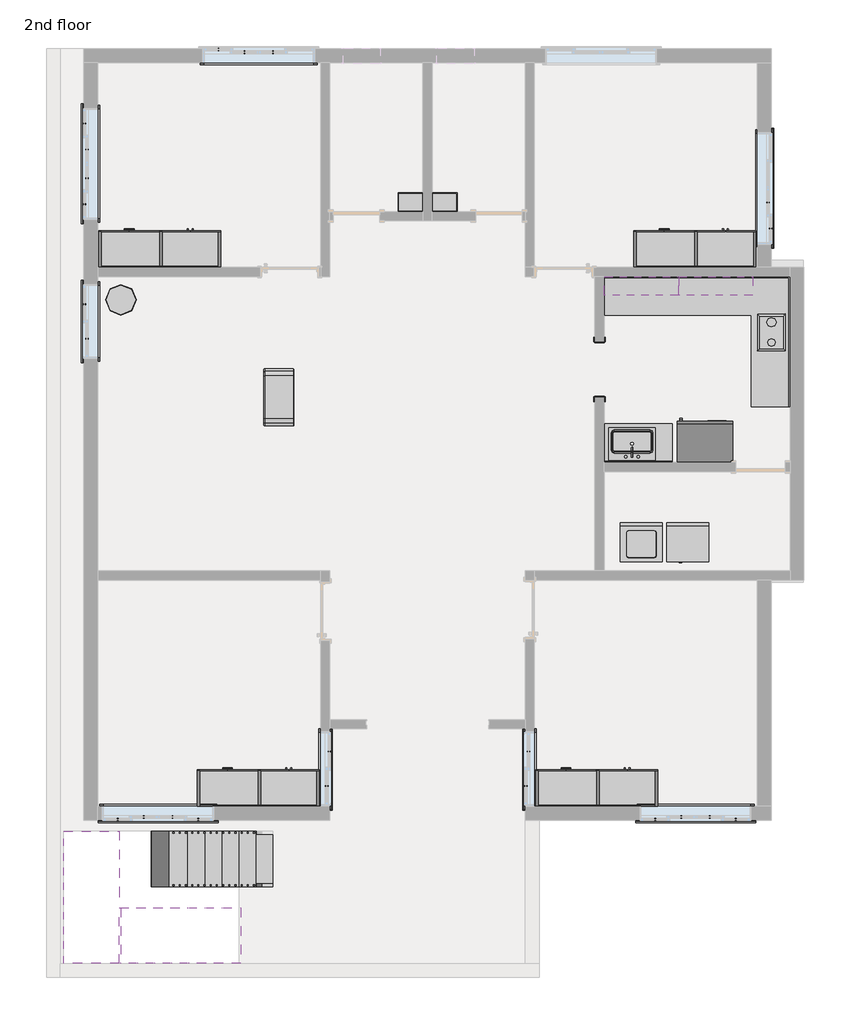
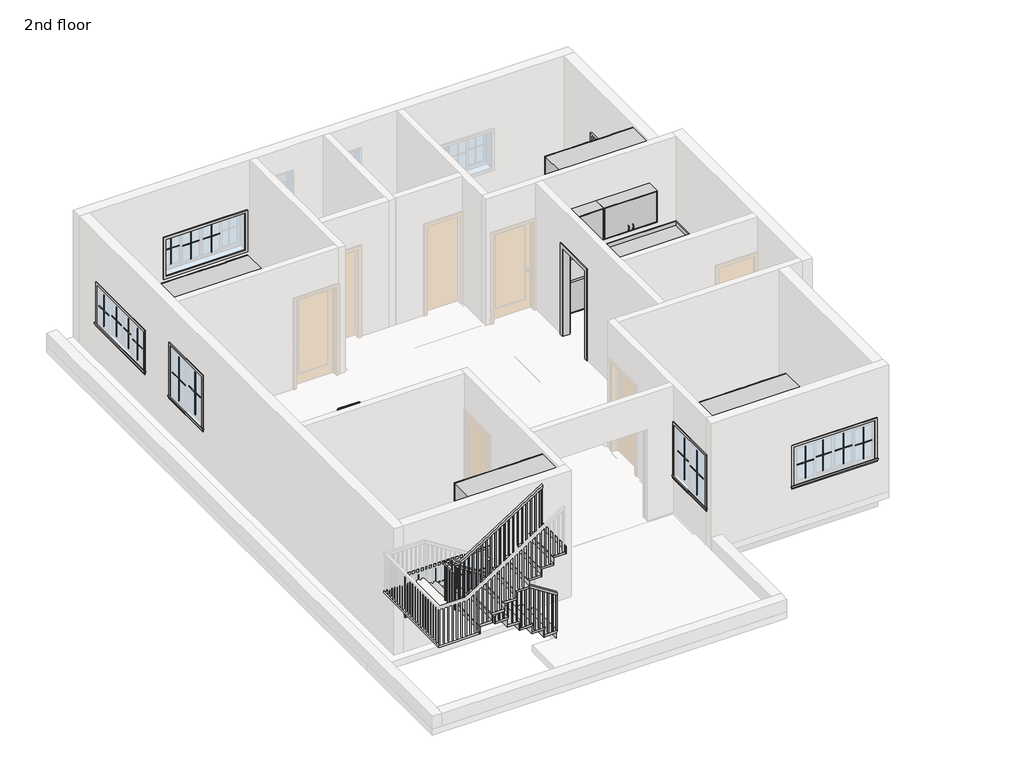
# One storey, part 3 of 4: 42 proxies, 15 furniture elements, 3 flow terminals, 2 stair flights, 1 railing, 1 slab.
"""IFC4 building model written with IfcOpenShell, lengths in millimetres."""

from ifc_helpers import new_model, si_unit, frame, origin, place, context, project, spatial, polyline, outline, extrude, faceted_brep, transform, mapped, element, save
from components import proxy_3c1fa1d0, proxy_97c73763, muntin_pattern_2x2_muntin_pattern_2x2_c2d27229, muntin_pattern_2x2_muntin_pattern_2x2_cf37b409, muntin_pattern_2x2_muntin_pattern_2x2_31a16349, proxy_7dd6dadb, trim_window_exterior_flat_with_sill_ac84ebb5, trim_window_exterior_flat_with_sill_7cfdd449, trim_window_exterior_flat_with_sill_3c945769, trim_window_interior_flat_picture_frame_caf2db4f, trim_window_interior_flat_picture_frame_f1e0b15b, trim_window_interior_flat_picture_frame_0edfbaa2, proxy_e75280ca, flow_terminal_7145266d, flow_terminal_4d548711, furniture_2dca108f, furniture_65fa61b5, furniture_1wardrobe_6271_1wardrobe_6271_4dd35231, furniture_3428e43d, furniture_bf8a676d, furniture_97fe820d, furniture_a6d59748, furniture_f5a42f9b, furniture_9d41381f, furniture_ea954fa4, non_monolithic_landing_bb243dde, stair_flight_4e768039, stair_flight_9d0467a4

model = new_model("IFC4")

# Units and contexts
model_context = context("Model", 3, world=origin())
ifc_project = project(units=[si_unit("LENGTHUNIT", "METRE", prefix="MILLI")], contexts=[model_context])

# Site, building, storey
site = spatial("IfcSite", under=ifc_project)
building = spatial("IfcBuilding", under=site)
storey = spatial("IfcBuildingStorey", under=building, Name="2nd floor", Elevation=7010.4)

# Proxies
placement = place(None, origin())
proxy_shape = proxy_3c1fa1d0(model_context)
element("IfcBuildingElementProxy", 1, Name="Cook Top-2 Unit : 12\" x 18\" 2", ObjectType="Cook Top-2 Unit : 12\" x 18\" 2", at=placement, inside=storey, context=model_context, shape_type="MappedRepresentation", body=[
    mapped(proxy_shape, transform((-1440.8124084, 5502.3713848, 7010.4), x_axis=(1.0, 0.0, 0.0), y_axis=(0.0, 1.0, 0.0), z_axis=(0.0, 0.0, 1.0))),
])
proxy_2_shape = proxy_97c73763(model_context)
element("IfcBuildingElementProxy", 2, Name="Dryer : 27\" x 25\" x 35\"", ObjectType="Dryer : 27\" x 25\" x 35\"", at=placement, inside=storey, context=model_context, shape_type="MappedRepresentation", body=[
    mapped(proxy_2_shape, transform((-3115.1998647, 1776.2351766, 7010.4), x_axis=(1.0, 0.0, 0.0), y_axis=(0.0, 1.0, 0.0), z_axis=(0.0, 0.0, 1.0))),
])
muntin_pattern_2x2_muntin_pattern_2x2_shape = muntin_pattern_2x2_muntin_pattern_2x2_c2d27229(model_context)
element("IfcBuildingElementProxy", 3, Name="Muntin Pattern_2x2 : Muntin Pattern_2x2", ObjectType="Muntin Pattern_2x2 : Muntin Pattern_2x2", at=placement, inside=storey, context=model_context, shape_type="MappedRepresentation", body=[
    mapped(muntin_pattern_2x2_muntin_pattern_2x2_shape, transform((-12588.2374084, 5426.2336804, 8007.35), x_axis=(0.0, -1.0, 0.0), y_axis=(1.0, 0.0, 0.0), z_axis=(0.0, 0.0, 1.0))),
])
element("IfcBuildingElementProxy", 4, Name="Muntin Pattern_2x2 : Muntin Pattern_2x2", ObjectType="Muntin Pattern_2x2 : Muntin Pattern_2x2", at=placement, inside=storey, context=model_context, shape_type="MappedRepresentation", body=[
    mapped(muntin_pattern_2x2_muntin_pattern_2x2_shape, transform((-12632.6874084, 5994.5586804, 8007.35), x_axis=(0.0, -1.0, 0.0), y_axis=(1.0, 0.0, 0.0), z_axis=(0.0, 0.0, 1.0))),
])
muntin_pattern_2x2_muntin_pattern_2x2_2_shape = muntin_pattern_2x2_muntin_pattern_2x2_cf37b409(model_context)
element("IfcBuildingElementProxy", 5, Name="Muntin Pattern_2x2 : Muntin Pattern_2x2", ObjectType="Muntin Pattern_2x2 : Muntin Pattern_2x2", at=placement, inside=storey, context=model_context, shape_type="MappedRepresentation", body=[
    mapped(muntin_pattern_2x2_muntin_pattern_2x2_2_shape, transform((-8657.5874084, -1908.0163196, 8007.35), x_axis=(0.0, -1.0, 0.0), y_axis=(1.0, 0.0, 0.0), z_axis=(0.0, 0.0, 1.0))),
])
element("IfcBuildingElementProxy", 6, Name="Muntin Pattern_2x2 : Muntin Pattern_2x2", ObjectType="Muntin Pattern_2x2 : Muntin Pattern_2x2", at=placement, inside=storey, context=model_context, shape_type="MappedRepresentation", body=[
    mapped(muntin_pattern_2x2_muntin_pattern_2x2_2_shape, transform((-8613.1374084, -1339.6913196, 8007.35), x_axis=(0.0, -1.0, 0.0), y_axis=(1.0, 0.0, 0.0), z_axis=(0.0, 0.0, 1.0))),
])
element("IfcBuildingElementProxy", 7, Name="Muntin Pattern_2x2 : Muntin Pattern_2x2", ObjectType="Muntin Pattern_2x2 : Muntin Pattern_2x2", at=placement, inside=storey, context=model_context, shape_type="MappedRepresentation", body=[
    mapped(muntin_pattern_2x2_muntin_pattern_2x2_2_shape, transform((-5349.2374084, -1339.6913196, 8007.35), x_axis=(0.0, 1.0, 0.0), y_axis=(-1.0, 0.0, 0.0), z_axis=(0.0, 0.0, 1.0))),
])
element("IfcBuildingElementProxy", 8, Name="Muntin Pattern_2x2 : Muntin Pattern_2x2", ObjectType="Muntin Pattern_2x2 : Muntin Pattern_2x2", at=placement, inside=storey, context=model_context, shape_type="MappedRepresentation", body=[
    mapped(muntin_pattern_2x2_muntin_pattern_2x2_2_shape, transform((-5393.6874084, -1908.0163196, 8007.35), x_axis=(0.0, 1.0, 0.0), y_axis=(-1.0, 0.0, 0.0), z_axis=(0.0, 0.0, 1.0))),
])
muntin_pattern_2x2_muntin_pattern_2x2_3_shape = muntin_pattern_2x2_muntin_pattern_2x2_31a16349(model_context)
element("IfcBuildingElementProxy", 9, Name="Muntin Pattern_2x2 : Muntin Pattern_2x2", ObjectType="Muntin Pattern_2x2 : Muntin Pattern_2x2", at=placement, inside=storey, context=model_context, shape_type="MappedRepresentation", body=[
    mapped(muntin_pattern_2x2_muntin_pattern_2x2_3_shape, transform((-10432.4124084, 10171.2711804, 8007.35), x_axis=(1.0, 0.0, 0.0), y_axis=(0.0, 1.0, 0.0), z_axis=(0.0, 0.0, 1.0))),
])
element("IfcBuildingElementProxy", 10, Name="Muntin Pattern_2x2 : Muntin Pattern_2x2", ObjectType="Muntin Pattern_2x2 : Muntin Pattern_2x2", at=placement, inside=storey, context=model_context, shape_type="MappedRepresentation", body=[
    mapped(muntin_pattern_2x2_muntin_pattern_2x2_3_shape, transform((-10006.9624084, 10126.8211804, 8007.35), x_axis=(1.0, 0.0, 0.0), y_axis=(0.0, 1.0, 0.0), z_axis=(0.0, 0.0, 1.0))),
])
element("IfcBuildingElementProxy", 11, Name="Muntin Pattern_2x2 : Muntin Pattern_2x2", ObjectType="Muntin Pattern_2x2 : Muntin Pattern_2x2", at=placement, inside=storey, context=model_context, shape_type="MappedRepresentation", body=[
    mapped(muntin_pattern_2x2_muntin_pattern_2x2_3_shape, transform((-9537.0624084, 10126.8211804, 8007.35), x_axis=(1.0, 0.0, 0.0), y_axis=(0.0, 1.0, 0.0), z_axis=(0.0, 0.0, 1.0))),
])
element("IfcBuildingElementProxy", 12, Name="Muntin Pattern_2x2 : Muntin Pattern_2x2", ObjectType="Muntin Pattern_2x2 : Muntin Pattern_2x2", at=placement, inside=storey, context=model_context, shape_type="MappedRepresentation", body=[
    mapped(muntin_pattern_2x2_muntin_pattern_2x2_3_shape, transform((-12632.6874084, 7634.4461804, 8007.35), x_axis=(0.0, 1.0, 0.0), y_axis=(-1.0, 0.0, 0.0), z_axis=(0.0, 0.0, 1.0))),
])
element("IfcBuildingElementProxy", 13, Name="Muntin Pattern_2x2 : Muntin Pattern_2x2", ObjectType="Muntin Pattern_2x2 : Muntin Pattern_2x2", at=placement, inside=storey, context=model_context, shape_type="MappedRepresentation", body=[
    mapped(muntin_pattern_2x2_muntin_pattern_2x2_3_shape, transform((-12588.2374084, 8059.8961804, 8007.35), x_axis=(0.0, 1.0, 0.0), y_axis=(-1.0, 0.0, 0.0), z_axis=(0.0, 0.0, 1.0))),
])
element("IfcBuildingElementProxy", 14, Name="Muntin Pattern_2x2 : Muntin Pattern_2x2", ObjectType="Muntin Pattern_2x2 : Muntin Pattern_2x2", at=placement, inside=storey, context=model_context, shape_type="MappedRepresentation", body=[
    mapped(muntin_pattern_2x2_muntin_pattern_2x2_3_shape, transform((-12588.2374084, 8529.7961804, 8007.35), x_axis=(0.0, 1.0, 0.0), y_axis=(-1.0, 0.0, 0.0), z_axis=(0.0, 0.0, 1.0))),
])
element("IfcBuildingElementProxy", 15, Name="Muntin Pattern_2x2 : Muntin Pattern_2x2", ObjectType="Muntin Pattern_2x2 : Muntin Pattern_2x2", at=placement, inside=storey, context=model_context, shape_type="MappedRepresentation", body=[
    mapped(muntin_pattern_2x2_muntin_pattern_2x2_3_shape, transform((-12632.6874084, 8955.2461804, 8007.35), x_axis=(0.0, 1.0, 0.0), y_axis=(-1.0, 0.0, 0.0), z_axis=(0.0, 0.0, 1.0))),
])
element("IfcBuildingElementProxy", 16, Name="Muntin Pattern_2x2 : Muntin Pattern_2x2", ObjectType="Muntin Pattern_2x2 : Muntin Pattern_2x2", at=placement, inside=storey, context=model_context, shape_type="MappedRepresentation", body=[
    mapped(muntin_pattern_2x2_muntin_pattern_2x2_3_shape, transform((-1418.5874084, 7659.8461804, 8007.35), x_axis=(0.0, -1.0, 0.0), y_axis=(1.0, 0.0, 0.0), z_axis=(0.0, 0.0, 1.0))),
])
element("IfcBuildingElementProxy", 17, Name="Muntin Pattern_2x2 : Muntin Pattern_2x2", ObjectType="Muntin Pattern_2x2 : Muntin Pattern_2x2", at=placement, inside=storey, context=model_context, shape_type="MappedRepresentation", body=[
    mapped(muntin_pattern_2x2_muntin_pattern_2x2_3_shape, transform((-1374.1374084, 7234.3961804, 8007.35), x_axis=(0.0, -1.0, 0.0), y_axis=(1.0, 0.0, 0.0), z_axis=(0.0, 0.0, 1.0))),
])
element("IfcBuildingElementProxy", 18, Name="Muntin Pattern_2x2 : Muntin Pattern_2x2", ObjectType="Muntin Pattern_2x2 : Muntin Pattern_2x2", at=placement, inside=storey, context=model_context, shape_type="MappedRepresentation", body=[
    mapped(muntin_pattern_2x2_muntin_pattern_2x2_3_shape, transform((-1948.8124084, -2458.8788196, 8007.35), x_axis=(-1.0, 0.0, 0.0), y_axis=(0.0, -1.0, 0.0), z_axis=(0.0, 0.0, 1.0))),
])
element("IfcBuildingElementProxy", 19, Name="Muntin Pattern_2x2 : Muntin Pattern_2x2", ObjectType="Muntin Pattern_2x2 : Muntin Pattern_2x2", at=placement, inside=storey, context=model_context, shape_type="MappedRepresentation", body=[
    mapped(muntin_pattern_2x2_muntin_pattern_2x2_3_shape, transform((-2374.2624084, -2414.4288196, 8007.35), x_axis=(-1.0, 0.0, 0.0), y_axis=(0.0, -1.0, 0.0), z_axis=(0.0, 0.0, 1.0))),
])
element("IfcBuildingElementProxy", 20, Name="Muntin Pattern_2x2 : Muntin Pattern_2x2", ObjectType="Muntin Pattern_2x2 : Muntin Pattern_2x2", at=placement, inside=storey, context=model_context, shape_type="MappedRepresentation", body=[
    mapped(muntin_pattern_2x2_muntin_pattern_2x2_3_shape, transform((-2844.1624084, -2414.4288196, 8007.35), x_axis=(-1.0, 0.0, 0.0), y_axis=(0.0, -1.0, 0.0), z_axis=(0.0, 0.0, 1.0))),
])
element("IfcBuildingElementProxy", 21, Name="Muntin Pattern_2x2 : Muntin Pattern_2x2", ObjectType="Muntin Pattern_2x2 : Muntin Pattern_2x2", at=placement, inside=storey, context=model_context, shape_type="MappedRepresentation", body=[
    mapped(muntin_pattern_2x2_muntin_pattern_2x2_3_shape, transform((-3269.6124084, -2458.8788196, 8007.35), x_axis=(-1.0, 0.0, 0.0), y_axis=(0.0, -1.0, 0.0), z_axis=(0.0, 0.0, 1.0))),
])
element("IfcBuildingElementProxy", 22, Name="Muntin Pattern_2x2 : Muntin Pattern_2x2", ObjectType="Muntin Pattern_2x2 : Muntin Pattern_2x2", at=placement, inside=storey, context=model_context, shape_type="MappedRepresentation", body=[
    mapped(muntin_pattern_2x2_muntin_pattern_2x2_3_shape, transform((-10762.6124084, -2458.8788196, 8007.35), x_axis=(-1.0, 0.0, 0.0), y_axis=(0.0, -1.0, 0.0), z_axis=(0.0, 0.0, 1.0))),
])
element("IfcBuildingElementProxy", 23, Name="Muntin Pattern_2x2 : Muntin Pattern_2x2", ObjectType="Muntin Pattern_2x2 : Muntin Pattern_2x2", at=placement, inside=storey, context=model_context, shape_type="MappedRepresentation", body=[
    mapped(muntin_pattern_2x2_muntin_pattern_2x2_3_shape, transform((-11188.0624084, -2414.4288196, 8007.35), x_axis=(-1.0, 0.0, 0.0), y_axis=(0.0, -1.0, 0.0), z_axis=(0.0, 0.0, 1.0))),
])
element("IfcBuildingElementProxy", 24, Name="Muntin Pattern_2x2 : Muntin Pattern_2x2", ObjectType="Muntin Pattern_2x2 : Muntin Pattern_2x2", at=placement, inside=storey, context=model_context, shape_type="MappedRepresentation", body=[
    mapped(muntin_pattern_2x2_muntin_pattern_2x2_3_shape, transform((-11657.9624084, -2414.4288196, 8007.35), x_axis=(-1.0, 0.0, 0.0), y_axis=(0.0, -1.0, 0.0), z_axis=(0.0, 0.0, 1.0))),
])
element("IfcBuildingElementProxy", 25, Name="Muntin Pattern_2x2 : Muntin Pattern_2x2", ObjectType="Muntin Pattern_2x2 : Muntin Pattern_2x2", at=placement, inside=storey, context=model_context, shape_type="MappedRepresentation", body=[
    mapped(muntin_pattern_2x2_muntin_pattern_2x2_3_shape, transform((-12083.4124084, -2458.8788196, 8007.35), x_axis=(-1.0, 0.0, 0.0), y_axis=(0.0, -1.0, 0.0), z_axis=(0.0, 0.0, 1.0))),
])
proxy_3_shape = proxy_7dd6dadb(model_context)
element("IfcBuildingElementProxy", 26, Name="Passage Opening-Cased : 36\" x 84\"", ObjectType="Passage Opening-Cased : 36\" x 84\"", at=placement, inside=storey, context=model_context, shape_type="MappedRepresentation", body=[
    mapped(proxy_3_shape, transform((-4184.0124084, 4931.1848371, 7010.4), x_axis=(0.0, 1.0, 0.0), y_axis=(-1.0, 0.0, 0.0), z_axis=(0.0, 0.0, 1.0))),
])
trim_window_exterior_flat_with_sill_shape = trim_window_exterior_flat_with_sill_ac84ebb5(model_context)
element("IfcBuildingElementProxy", 27, Name="Trim-Window-Exterior-Flat : with Sill", ObjectType="Trim-Window-Exterior-Flat : with Sill", at=placement, inside=storey, context=model_context, shape_type="MappedRepresentation", body=[
    mapped(trim_window_exterior_flat_with_sill_shape, transform((-12642.2124084, 5710.3961804, 9144.0), x_axis=(0.0, 1.0, 0.0), y_axis=(0.0, 0.0, -1.0), z_axis=(-1.0, 0.0, 0.0))),
])
trim_window_exterior_flat_with_sill_2_shape = trim_window_exterior_flat_with_sill_7cfdd449(model_context)
element("IfcBuildingElementProxy", 28, Name="Trim-Window-Exterior-Flat : with Sill", ObjectType="Trim-Window-Exterior-Flat : with Sill", at=placement, inside=storey, context=model_context, shape_type="MappedRepresentation", body=[
    mapped(trim_window_exterior_flat_with_sill_2_shape, transform((-8603.6124084, -1623.8538196, 9144.0), x_axis=(0.0, 1.0, 0.0), y_axis=(0.0, 0.0, 1.0), z_axis=(1.0, 0.0, 0.0))),
])
element("IfcBuildingElementProxy", 29, Name="Trim-Window-Exterior-Flat : with Sill", ObjectType="Trim-Window-Exterior-Flat : with Sill", at=placement, inside=storey, context=model_context, shape_type="MappedRepresentation", body=[
    mapped(trim_window_exterior_flat_with_sill_2_shape, transform((-5403.2124084, -1623.8538196, 9144.0), x_axis=(0.0, -1.0, 0.0), y_axis=(0.0, 0.0, 1.0), z_axis=(-1.0, 0.0, 0.0))),
])
trim_window_exterior_flat_with_sill_3_shape = trim_window_exterior_flat_with_sill_3c945769(model_context)
element("IfcBuildingElementProxy", 30, Name="Trim-Window-Exterior-Flat : with Sill", ObjectType="Trim-Window-Exterior-Flat : with Sill", at=placement, inside=storey, context=model_context, shape_type="MappedRepresentation", body=[
    mapped(trim_window_exterior_flat_with_sill_3_shape, transform((-12642.2124084, 8294.8461804, 8839.2), x_axis=(0.0, -1.0, 0.0), y_axis=(0.0, 0.0, 1.0), z_axis=(-1.0, 0.0, 0.0))),
])
element("IfcBuildingElementProxy", 31, Name="Trim-Window-Exterior-Flat : with Sill", ObjectType="Trim-Window-Exterior-Flat : with Sill", at=placement, inside=storey, context=model_context, shape_type="MappedRepresentation", body=[
    mapped(trim_window_exterior_flat_with_sill_3_shape, transform((-1364.6124084, 7894.7961804, 8839.2), x_axis=(0.0, 1.0, 0.0), y_axis=(0.0, 0.0, 1.0), z_axis=(1.0, 0.0, 0.0))),
])
element("IfcBuildingElementProxy", 32, Name="Trim-Window-Exterior-Flat : with Sill", ObjectType="Trim-Window-Exterior-Flat : with Sill", at=placement, inside=storey, context=model_context, shape_type="MappedRepresentation", body=[
    mapped(trim_window_exterior_flat_with_sill_3_shape, transform((-2609.2124084, -2468.4038196, 8839.2), x_axis=(1.0, 0.0, 0.0), y_axis=(0.0, 0.0, 1.0), z_axis=(0.0, -1.0, 0.0))),
])
element("IfcBuildingElementProxy", 33, Name="Trim-Window-Exterior-Flat : with Sill", ObjectType="Trim-Window-Exterior-Flat : with Sill", at=placement, inside=storey, context=model_context, shape_type="MappedRepresentation", body=[
    mapped(trim_window_exterior_flat_with_sill_3_shape, transform((-11423.0124084, -2468.4038196, 8839.2), x_axis=(1.0, 0.0, 0.0), y_axis=(0.0, 0.0, 1.0), z_axis=(0.0, -1.0, 0.0))),
])
trim_window_interior_flat_picture_frame_shape = trim_window_interior_flat_picture_frame_caf2db4f(model_context)
element("IfcBuildingElementProxy", 34, Name="Trim-Window-Interior-Flat : Picture Frame", ObjectType="Trim-Window-Interior-Flat : Picture Frame", at=placement, inside=storey, context=model_context, shape_type="MappedRepresentation", body=[
    mapped(trim_window_interior_flat_picture_frame_shape, transform((-12413.6124084, 5710.3961804, 9144.0), x_axis=(0.0, -1.0, 0.0), y_axis=(0.0, 0.0, -1.0), z_axis=(1.0, 0.0, 0.0))),
])
trim_window_interior_flat_picture_frame_2_shape = trim_window_interior_flat_picture_frame_f1e0b15b(model_context)
element("IfcBuildingElementProxy", 35, Name="Trim-Window-Interior-Flat : Picture Frame", ObjectType="Trim-Window-Interior-Flat : Picture Frame", at=placement, inside=storey, context=model_context, shape_type="MappedRepresentation", body=[
    mapped(trim_window_interior_flat_picture_frame_2_shape, transform((-8756.0124084, -1623.8538196, 9144.0), x_axis=(0.0, -1.0, 0.0), y_axis=(0.0, 0.0, 1.0), z_axis=(-1.0, 0.0, 0.0))),
])
element("IfcBuildingElementProxy", 36, Name="Trim-Window-Interior-Flat : Picture Frame", ObjectType="Trim-Window-Interior-Flat : Picture Frame", at=placement, inside=storey, context=model_context, shape_type="MappedRepresentation", body=[
    mapped(trim_window_interior_flat_picture_frame_2_shape, transform((-5250.8124084, -1623.8538196, 9144.0), x_axis=(0.0, 1.0, 0.0), y_axis=(0.0, 0.0, 1.0), z_axis=(1.0, 0.0, 0.0))),
])
trim_window_interior_flat_picture_frame_3_shape = trim_window_interior_flat_picture_frame_0edfbaa2(model_context)
element("IfcBuildingElementProxy", 37, Name="Trim-Window-Interior-Flat : Picture Frame", ObjectType="Trim-Window-Interior-Flat : Picture Frame", at=placement, inside=storey, context=model_context, shape_type="MappedRepresentation", body=[
    mapped(trim_window_interior_flat_picture_frame_3_shape, transform((-9772.0124084, 9952.1961804, 8839.2), x_axis=(1.0, 0.0, 0.0), y_axis=(0.0, 0.0, 1.0), z_axis=(0.0, -1.0, 0.0))),
])
element("IfcBuildingElementProxy", 38, Name="Trim-Window-Interior-Flat : Picture Frame", ObjectType="Trim-Window-Interior-Flat : Picture Frame", at=placement, inside=storey, context=model_context, shape_type="MappedRepresentation", body=[
    mapped(trim_window_interior_flat_picture_frame_3_shape, transform((-12413.6124084, 8294.8461804, 8839.2), x_axis=(0.0, 1.0, 0.0), y_axis=(0.0, 0.0, 1.0), z_axis=(1.0, 0.0, 0.0))),
])
element("IfcBuildingElementProxy", 39, Name="Trim-Window-Interior-Flat : Picture Frame", ObjectType="Trim-Window-Interior-Flat : Picture Frame", at=placement, inside=storey, context=model_context, shape_type="MappedRepresentation", body=[
    mapped(trim_window_interior_flat_picture_frame_3_shape, transform((-1593.2124084, 7894.7961804, 8839.2), x_axis=(0.0, -1.0, 0.0), y_axis=(0.0, 0.0, 1.0), z_axis=(-1.0, 0.0, 0.0))),
])
element("IfcBuildingElementProxy", 40, Name="Trim-Window-Interior-Flat : Picture Frame", ObjectType="Trim-Window-Interior-Flat : Picture Frame", at=placement, inside=storey, context=model_context, shape_type="MappedRepresentation", body=[
    mapped(trim_window_interior_flat_picture_frame_3_shape, transform((-2609.2124084, -2239.8038196, 8839.2), x_axis=(-1.0, 0.0, 0.0), y_axis=(0.0, 0.0, 1.0), z_axis=(0.0, 1.0, 0.0))),
])
element("IfcBuildingElementProxy", 41, Name="Trim-Window-Interior-Flat : Picture Frame", ObjectType="Trim-Window-Interior-Flat : Picture Frame", at=placement, inside=storey, context=model_context, shape_type="MappedRepresentation", body=[
    mapped(trim_window_interior_flat_picture_frame_3_shape, transform((-11423.0124084, -2239.8038196, 8839.2), x_axis=(-1.0, 0.0, 0.0), y_axis=(0.0, 0.0, 1.0), z_axis=(0.0, 1.0, 0.0))),
])
proxy_4_shape = proxy_e75280ca(model_context)
element("IfcBuildingElementProxy", 42, Name="Washer : 27\" x 25\" x 35\"", ObjectType="Washer : 27\" x 25\" x 35\"", at=placement, inside=storey, context=model_context, shape_type="MappedRepresentation", body=[
    mapped(proxy_4_shape, transform((-3918.6298768, 1811.7466156, 7010.4), x_axis=(1.0, 0.0, 0.0), y_axis=(0.0, 1.0, 0.0), z_axis=(0.0, 0.0, 1.0))),
])

# Flow terminals
flow_terminal_shape = flow_terminal_7145266d(model_context)
element("IfcFlowTerminal", 43, ObjectType="Sink - Work : 20\"x18\" 2", at=placement, inside=storey, context=model_context, shape_type="MappedRepresentation", body=[
    mapped(flow_terminal_shape, transform((-7282.8124084, 7513.7961804, 7924.8), x_axis=(-1.0, 0.0, 0.0), y_axis=(0.0, -1.0, 0.0), z_axis=(0.0, 0.0, 1.0))),
])
element("IfcFlowTerminal", 44, ObjectType="Sink - Work : 20\"x18\" 2", at=placement, inside=storey, context=model_context, shape_type="MappedRepresentation", body=[
    mapped(flow_terminal_shape, transform((-6724.0124084, 7513.7961804, 7924.8), x_axis=(-1.0, 0.0, 0.0), y_axis=(0.0, -1.0, 0.0), z_axis=(0.0, 0.0, 1.0))),
])
flow_terminal_2_shape = flow_terminal_4d548711(model_context)
element("IfcFlowTerminal", 45, ObjectType="Sink Kitchen-Single : 30\" x 21\"", at=placement, inside=storey, context=model_context, shape_type="MappedRepresentation", body=[
    mapped(flow_terminal_2_shape, transform((-3634.9231678, 3706.1415815, 7010.4), x_axis=(-1.0, 0.0, 0.0), y_axis=(0.0, -1.0, 0.0), z_axis=(0.0, 0.0, 1.0))),
])

# Furniture
furniture_shape = furniture_2dca108f(model_context)
element("IfcFurniture", 46, at=placement, inside=storey, context=model_context, shape_type="MappedRepresentation", body=[
    mapped(furniture_shape, transform((-9441.8124084, 4465.7961804, 7010.4), x_axis=(1.0, 0.0, 0.0), y_axis=(0.0, 1.0, 0.0), z_axis=(0.0, 0.0, 1.0))),
])
furniture_2_shape = furniture_65fa61b5(model_context)
element("IfcFurniture", 47, at=placement, inside=storey, context=model_context, shape_type="MappedRepresentation", body=[
    mapped(furniture_2_shape, transform((-3066.4124084, 3411.6961804, 7010.4), x_axis=(-1.0, 0.0, 0.0), y_axis=(0.0, -1.0, 0.0), z_axis=(0.0, 0.0, 1.0))),
])
furniture_1wardrobe_6271_1wardrobe_6271_shape = furniture_1wardrobe_6271_1wardrobe_6271_4dd35231(model_context)
element("IfcFurniture", 48, ObjectType="1Wardrobe_6271 : 1Wardrobe_6271", at=placement, inside=storey, context=model_context, shape_type="MappedRepresentation", body=[
    mapped(furniture_1wardrobe_6271_1wardrobe_6271_shape, transform((-10394.3124084, 6599.3961804, 7010.4), x_axis=(-1.0, 0.0, 0.0), y_axis=(0.0, -1.0, 0.0), z_axis=(0.0, 0.0, 1.0))),
])
element("IfcFurniture", 49, ObjectType="1Wardrobe_6271 : 1Wardrobe_6271", at=placement, inside=storey, context=model_context, shape_type="MappedRepresentation", body=[
    mapped(furniture_1wardrobe_6271_1wardrobe_6271_shape, transform((-1618.6124084, 6599.3961804, 7010.4), x_axis=(-1.0, 0.0, 0.0), y_axis=(0.0, -1.0, 0.0), z_axis=(0.0, 0.0, 1.0))),
])
element("IfcFurniture", 50, ObjectType="1Wardrobe_6271 : 1Wardrobe_6271", at=placement, inside=storey, context=model_context, shape_type="MappedRepresentation", body=[
    mapped(furniture_1wardrobe_6271_1wardrobe_6271_shape, transform((-3231.5124084, -2239.8038196, 7010.4), x_axis=(-1.0, 0.0, 0.0), y_axis=(0.0, -1.0, 0.0), z_axis=(0.0, 0.0, 1.0))),
])
element("IfcFurniture", 51, ObjectType="1Wardrobe_6271 : 1Wardrobe_6271", at=placement, inside=storey, context=model_context, shape_type="MappedRepresentation", body=[
    mapped(furniture_1wardrobe_6271_1wardrobe_6271_shape, transform((-8781.4124084, -2239.8038196, 7010.4), x_axis=(-1.0, 0.0, 0.0), y_axis=(0.0, -1.0, 0.0), z_axis=(0.0, 0.0, 1.0))),
])
furniture_3_shape = furniture_3428e43d(model_context)
element("IfcFurniture", 52, ObjectType="48\" 2", at=placement, inside=storey, context=model_context, shape_type="MappedRepresentation", body=[
    mapped(furniture_3_shape, transform((-2674.6573683, 6446.9961804, 7010.4), x_axis=(1.0, 0.0, 0.0), y_axis=(0.0, 1.0, 0.0), z_axis=(0.0, 0.0, 1.0))),
])
element("IfcFurniture", 53, ObjectType="48\" 3", at=placement, inside=storey, context=model_context, shape_type="MappedRepresentation", body=[
    mapped(furniture_3_shape, transform((-1059.8124084, 5013.8411403, 7010.4), x_axis=(0.0, -1.0, 0.0), y_axis=(1.0, 0.0, 0.0), z_axis=(0.0, 0.0, 1.0))),
])
furniture_4_shape = furniture_bf8a676d(model_context)
element("IfcFurniture", 54, ObjectType="Base Cabinet-Combo01 : 30\" 2", at=placement, inside=storey, context=model_context, shape_type="MappedRepresentation", body=[
    mapped(furniture_4_shape, transform((-3669.3501133, 6446.9961804, 7010.4), x_axis=(1.0, 0.0, 0.0), y_axis=(0.0, 1.0, 0.0), z_axis=(0.0, 0.0, 1.0))),
])
furniture_5_shape = furniture_97fe820d(model_context)
element("IfcFurniture", 55, ObjectType="Base Cabinet-Corner Unit-Square : 36\"", at=placement, inside=storey, context=model_context, shape_type="MappedRepresentation", body=[
    mapped(furniture_5_shape, transform((-1586.5501133, 6446.9961804, 7010.4), x_axis=(1.0, 0.0, 0.0), y_axis=(0.0, 1.0, 0.0), z_axis=(0.0, 0.0, 1.0))),
])
furniture_6_shape = furniture_a6d59748(model_context)
element("IfcFurniture", 56, ObjectType="Counter Top w Sink Hole : 24\" Depth", at=placement, inside=storey, context=model_context, shape_type="MappedRepresentation", body=[
    mapped(furniture_6_shape, transform((-4190.6747034, 3398.9961804, 7010.4), x_axis=(-1.0, 0.0, 0.0), y_axis=(0.0, -1.0, 0.0), z_axis=(0.0, 0.0, 1.0))),
])
furniture_7_shape = furniture_f5a42f9b(model_context)
element("IfcFurniture", 57, ObjectType="Counter Top-L Shaped : 24\" Depth", at=placement, inside=storey, context=model_context, shape_type="MappedRepresentation", body=[
    mapped(furniture_7_shape, transform((-1059.8124084, 5246.5338853, 7010.4), x_axis=(0.0, -1.0, 0.0), y_axis=(1.0, 0.0, 0.0), z_axis=(0.0, 0.0, 1.0))),
])
furniture_8_shape = furniture_9d41381f(model_context)
element("IfcFurniture", 58, ObjectType="Table-Trio End : 20\" Diameter", at=placement, inside=storey, context=model_context, shape_type="MappedRepresentation", body=[
    mapped(furniture_8_shape, transform((-12032.6124084, 6065.9961804, 7010.4), x_axis=(1.0, 0.0, 0.0), y_axis=(0.0, 1.0, 0.0), z_axis=(0.0, 0.0, 1.0))),
])
furniture_9_shape = furniture_ea954fa4(model_context)
element("IfcFurniture", 59, ObjectType="Upper Cabinet-Pass-Thru : 48\" x 30\" x 12\"", at=placement, inside=storey, context=model_context, shape_type="MappedRepresentation", body=[
    mapped(furniture_9_shape, transform((-3516.9501133, 6446.9961804, 7010.4), x_axis=(1.0, 0.0, 0.0), y_axis=(0.0, 1.0, 0.0), z_axis=(0.0, 0.0, 1.0))),
])
element("IfcFurniture", 60, ObjectType="Upper Cabinet-Pass-Thru : 48\" x 30\" x 12\"", at=placement, inside=storey, context=model_context, shape_type="MappedRepresentation", body=[
    mapped(furniture_9_shape, transform((-2297.7501133, 6446.9961804, 7010.4), x_axis=(1.0, 0.0, 0.0), y_axis=(0.0, 1.0, 0.0), z_axis=(0.0, 0.0, 1.0))),
])

# Railing
element("IfcRailing", 61, ObjectType="Handrail - Rectangular", at=placement, inside=storey, context=model_context, shape_type="SolidModel", body=[
    faceted_brep([(-9543.8120641, -3562.3669819, 8102.6), (-9543.8120641, -3562.3669819, 8042.386276), (-9543.8120641, -3511.5669819, 8042.386276), (-9543.8120641, -3511.5669819, 8102.6), (-11982.2120641, -3562.3669819, 9654.3090909), (-12033.0120641, -3562.3669819, 9626.4226396), (-12033.0120641, -3511.5669819, 9626.4226396), (-11982.2120641, -3511.5669819, 9654.3090909), (-11982.2120641, -3562.3669819, 9702.8), (-12033.0120641, -3562.3669819, 9652.0), (-12033.0120641, -3511.5669819, 9652.0), (-11982.2120641, -3511.5669819, 9702.8), (-12058.4120641, -3562.3669819, 9702.8), (-12058.4120641, -3562.3669819, 9652.0), (-12109.2120641, -3511.5669819, 9652.0), (-12109.2120641, -3511.5669819, 9702.8), (-12058.4120641, -3638.5669819, 9702.8), (-12058.4120641, -3638.5669819, 9652.0), (-12109.2120641, -3638.5669819, 9652.0), (-12109.2120641, -3638.5669819, 9702.8), (-12058.4120641, -3827.3038196, 9702.8), (-12058.4120641, -3878.1038196, 9652.0), (-12109.2120641, -3878.1038196, 9652.0), (-12109.2120641, -3827.3038196, 9702.8), (-12058.4120641, -3827.3038196, 9929.0909091), (-12058.4120641, -3878.1038196, 9878.2909091), (-12109.2120641, -3878.1038196, 9878.2909091), (-12109.2120641, -3827.3038196, 9929.0909091), (-12058.4120641, -3903.5038196, 9929.0909091), (-12058.4120641, -3903.5038196, 9878.2909091), (-12109.2120641, -3954.3038196, 9878.2909091), (-12109.2120641, -3954.3038196, 9929.0909091), (-11982.2120641, -3903.5038196, 9929.0909091), (-11967.4190691, -3903.5038196, 9878.2909091), (-11967.4190691, -3954.3038196, 9878.2909091), (-11982.2120641, -3954.3038196, 9929.0909091), (-10102.6120641, -3903.5038196, 11125.2), (-10102.6120641, -3954.3038196, 11125.2), (-10102.6120641, -3954.3038196, 11064.986276), (-10102.6120641, -3903.5038196, 11064.986276)], [[[0, 1, 2, 3]], [[1, 0, 4, 5]], [[2, 1, 5, 6]], [[3, 2, 6, 7]], [[0, 3, 7, 4]], [[5, 4, 8, 9]], [[6, 5, 9, 10]], [[7, 6, 10, 11]], [[4, 7, 11, 8]], [[9, 8, 12, 13]], [[10, 9, 13, 14]], [[11, 10, 14, 15]], [[8, 11, 15, 12]], [[13, 12, 16, 17]], [[14, 13, 17, 18]], [[15, 14, 18, 19]], [[12, 15, 19, 16]], [[17, 16, 20, 21]], [[18, 17, 21, 22]], [[19, 18, 22, 23]], [[16, 19, 23, 20]], [[21, 20, 24, 25]], [[22, 21, 25, 26]], [[23, 22, 26, 27]], [[20, 23, 27, 24]], [[25, 24, 28, 29]], [[26, 25, 29, 30]], [[27, 26, 30, 31]], [[24, 27, 31, 28]], [[29, 28, 32, 33]], [[30, 29, 33, 34]], [[31, 30, 34, 35]], [[28, 31, 35, 32]], [[36, 37, 38, 39]], [[33, 32, 36, 39]], [[34, 33, 39, 38]], [[35, 34, 38, 37]], [[32, 35, 37, 36]]]),
    extrude(outline(polyline([(11026.5976396, -10162.9370641), (10033.0, -10162.9370641), (10033.0, -10143.8870641), (11038.7203669, -10143.8870641), (11026.5976396, -10162.9370641)])), frame((0.0, -3938.4288196, 0.0), z_axis=(0.0, 1.0, 0.0), x_axis=(0.0, 0.0, 1.0)), (0.0, 0.0, 1.0), 19.05),
    extrude(outline(polyline([(10961.9430941, -10264.5370641), (10033.0, -10264.5370641), (10033.0, -10245.4870641), (10974.0658214, -10245.4870641), (10961.9430941, -10264.5370641)])), frame((0.0, -3938.4288196, 0.0), z_axis=(0.0, 1.0, 0.0), x_axis=(0.0, 0.0, 1.0)), (0.0, 0.0, 1.0), 19.05),
    extrude(outline(polyline([(10897.2885487, -10366.1370641), (10033.0, -10366.1370641), (10033.0, -10347.0870641), (10909.411276, -10347.0870641), (10897.2885487, -10366.1370641)])), frame((0.0, -3938.4288196, 0.0), z_axis=(0.0, 1.0, 0.0), x_axis=(0.0, 0.0, 1.0)), (0.0, 0.0, 1.0), 19.05),
    extrude(outline(polyline([(10832.6340032, -10467.7370641), (9855.2, -10467.7370641), (9855.2, -10448.6870641), (10844.7567305, -10448.6870641), (10832.6340032, -10467.7370641)])), frame((0.0, -3938.4288196, 0.0), z_axis=(0.0, 1.0, 0.0), x_axis=(0.0, 0.0, 1.0)), (0.0, 0.0, 1.0), 19.05),
    extrude(outline(polyline([(10767.9794578, -10569.3370641), (9855.2, -10569.3370641), (9855.2, -10550.2870641), (10780.1021851, -10550.2870641), (10767.9794578, -10569.3370641)])), frame((0.0, -3938.4288196, 0.0), z_axis=(0.0, 1.0, 0.0), x_axis=(0.0, 0.0, 1.0)), (0.0, 0.0, 1.0), 19.05),
    extrude(outline(polyline([(10703.3249123, -10670.9370641), (9855.2, -10670.9370641), (9855.2, -10651.8870641), (10715.4476396, -10651.8870641), (10703.3249123, -10670.9370641)])), frame((0.0, -3938.4288196, 0.0), z_axis=(0.0, 1.0, 0.0), x_axis=(0.0, 0.0, 1.0)), (0.0, 0.0, 1.0), 19.05),
    extrude(outline(polyline([(10638.6703669, -10772.5370641), (9677.4, -10772.5370641), (9677.4, -10753.4870641), (10650.7930941, -10753.4870641), (10638.6703669, -10772.5370641)])), frame((0.0, -3938.4288196, 0.0), z_axis=(0.0, 1.0, 0.0), x_axis=(0.0, 0.0, 1.0)), (0.0, 0.0, 1.0), 19.05),
    extrude(outline(polyline([(10574.0158214, -10874.1370641), (9677.4, -10874.1370641), (9677.4, -10855.0870641), (10586.1385487, -10855.0870641), (10574.0158214, -10874.1370641)])), frame((0.0, -3938.4288196, 0.0), z_axis=(0.0, 1.0, 0.0), x_axis=(0.0, 0.0, 1.0)), (0.0, 0.0, 1.0), 19.05),
    extrude(outline(polyline([(10509.361276, -10975.7370641), (9499.6, -10975.7370641), (9499.6, -10956.6870641), (10521.4840032, -10956.6870641), (10509.361276, -10975.7370641)])), frame((0.0, -3938.4288196, 0.0), z_axis=(0.0, 1.0, 0.0), x_axis=(0.0, 0.0, 1.0)), (0.0, 0.0, 1.0), 19.05),
    extrude(outline(polyline([(10444.7067305, -11077.3370641), (9499.6, -11077.3370641), (9499.6, -11058.2870641), (10456.8294578, -11058.2870641), (10444.7067305, -11077.3370641)])), frame((0.0, -3938.4288196, 0.0), z_axis=(0.0, 1.0, 0.0), x_axis=(0.0, 0.0, 1.0)), (0.0, 0.0, 1.0), 19.05),
    extrude(outline(polyline([(10380.0521851, -11178.9370641), (9499.6, -11178.9370641), (9499.6, -11159.8870641), (10392.1749123, -11159.8870641), (10380.0521851, -11178.9370641)])), frame((0.0, -3938.4288196, 0.0), z_axis=(0.0, 1.0, 0.0), x_axis=(0.0, 0.0, 1.0)), (0.0, 0.0, 1.0), 19.05),
    extrude(outline(polyline([(10315.3976396, -11280.5370641), (9321.8, -11280.5370641), (9321.8, -11261.4870641), (10327.5203669, -11261.4870641), (10315.3976396, -11280.5370641)])), frame((0.0, -3938.4288196, 0.0), z_axis=(0.0, 1.0, 0.0), x_axis=(0.0, 0.0, 1.0)), (0.0, 0.0, 1.0), 19.05),
    extrude(outline(polyline([(10250.7430941, -11382.1370641), (9321.8, -11382.1370641), (9321.8, -11363.0870641), (10262.8658214, -11363.0870641), (10250.7430941, -11382.1370641)])), frame((0.0, -3938.4288196, 0.0), z_axis=(0.0, 1.0, 0.0), x_axis=(0.0, 0.0, 1.0)), (0.0, 0.0, 1.0), 19.05),
    extrude(outline(polyline([(10186.0885487, -11483.7370641), (9321.8, -11483.7370641), (9321.8, -11464.6870641), (10198.211276, -11464.6870641), (10186.0885487, -11483.7370641)])), frame((0.0, -3938.4288196, 0.0), z_axis=(0.0, 1.0, 0.0), x_axis=(0.0, 0.0, 1.0)), (0.0, 0.0, 1.0), 19.05),
    extrude(outline(polyline([(10121.4340032, -11585.3370641), (9144.0, -11585.3370641), (9144.0, -11566.2870641), (10133.5567305, -11566.2870641), (10121.4340032, -11585.3370641)])), frame((0.0, -3938.4288196, 0.0), z_axis=(0.0, 1.0, 0.0), x_axis=(0.0, 0.0, 1.0)), (0.0, 0.0, 1.0), 19.05),
    extrude(outline(polyline([(10056.7794578, -11686.9370641), (9144.0, -11686.9370641), (9144.0, -11667.8870641), (10068.9021851, -11667.8870641), (10056.7794578, -11686.9370641)])), frame((0.0, -3938.4288196, 0.0), z_axis=(0.0, 1.0, 0.0), x_axis=(0.0, 0.0, 1.0)), (0.0, 0.0, 1.0), 19.05),
    extrude(outline(polyline([(9992.1249123, -11788.5370641), (9144.0, -11788.5370641), (9144.0, -11769.4870641), (10004.2476396, -11769.4870641), (9992.1249123, -11788.5370641)])), frame((0.0, -3938.4288196, 0.0), z_axis=(0.0, 1.0, 0.0), x_axis=(0.0, 0.0, 1.0)), (0.0, 0.0, 1.0), 19.05),
    extrude(outline(polyline([(9927.4703669, -11890.1370641), (8966.2, -11890.1370641), (8966.2, -11871.0870641), (9939.5930941, -11871.0870641), (9927.4703669, -11890.1370641)])), frame((0.0, -3938.4288196, 0.0), z_axis=(0.0, 1.0, 0.0), x_axis=(0.0, 0.0, 1.0)), (0.0, 0.0, 1.0), 19.05),
    extrude(outline(polyline([(9862.8158214, -11991.7370641), (8966.2, -11991.7370641), (8966.2, -11972.6870641), (9874.9385487, -11972.6870641), (9862.8158214, -11991.7370641)])), frame((0.0, -3938.4288196, 0.0), z_axis=(0.0, 1.0, 0.0), x_axis=(0.0, 0.0, 1.0)), (0.0, 0.0, 1.0), 19.05),
    extrude(outline(polyline([(-12074.2870641, -3832.2419819), (-12074.2870641, -3851.2919819), (-12093.3370641, -3851.2919819), (-12093.3370641, -3832.2419819), (-12074.2870641, -3832.2419819)])), frame((0.0, 0.0, 8788.4), z_axis=(0.0, 0.0, 1.0), x_axis=(1.0, 0.0, 0.0)), (0.0, 0.0, 1.0), 1089.8909091),
    extrude(outline(polyline([(-12074.2870641, -3730.6419819), (-12074.2870641, -3749.6919819), (-12093.3370641, -3749.6919819), (-12093.3370641, -3730.6419819), (-12074.2870641, -3730.6419819)])), frame((0.0, 0.0, 8788.4), z_axis=(0.0, 0.0, 1.0), x_axis=(1.0, 0.0, 0.0)), (0.0, 0.0, 1.0), 863.6),
    extrude(outline(polyline([(-12074.2870641, -3629.0419819), (-12074.2870641, -3648.0919819), (-12093.3370641, -3648.0919819), (-12093.3370641, -3629.0419819), (-12074.2870641, -3629.0419819)])), frame((0.0, 0.0, 8788.4), z_axis=(0.0, 0.0, 1.0), x_axis=(1.0, 0.0, 0.0)), (0.0, 0.0, 1.0), 863.6),
    extrude(outline(polyline([(9600.1567305, -11991.7370641), (8610.6, -11991.7370641), (8610.6, -11972.6870641), (9588.0340032, -11972.6870641), (9600.1567305, -11991.7370641)])), frame((0.0, -3546.4919819, 0.0), z_axis=(0.0, 1.0, 0.0), x_axis=(0.0, 0.0, 1.0)), (0.0, 0.0, 1.0), 19.05),
    extrude(outline(polyline([(9535.5021851, -11890.1370641), (8610.6, -11890.1370641), (8610.6, -11871.0870641), (9523.3794578, -11871.0870641), (9535.5021851, -11890.1370641)])), frame((0.0, -3546.4919819, 0.0), z_axis=(0.0, 1.0, 0.0), x_axis=(0.0, 0.0, 1.0)), (0.0, 0.0, 1.0), 19.05),
    extrude(outline(polyline([(9470.8476396, -11788.5370641), (8610.6, -11788.5370641), (8610.6, -11769.4870641), (9458.7249123, -11769.4870641), (9470.8476396, -11788.5370641)])), frame((0.0, -3546.4919819, 0.0), z_axis=(0.0, 1.0, 0.0), x_axis=(0.0, 0.0, 1.0)), (0.0, 0.0, 1.0), 19.05),
    extrude(outline(polyline([(9406.1930941, -11686.9370641), (8432.8, -11686.9370641), (8432.8, -11667.8870641), (9394.0703669, -11667.8870641), (9406.1930941, -11686.9370641)])), frame((0.0, -3546.4919819, 0.0), z_axis=(0.0, 1.0, 0.0), x_axis=(0.0, 0.0, 1.0)), (0.0, 0.0, 1.0), 19.05),
    extrude(outline(polyline([(9341.5385487, -11585.3370641), (8432.8, -11585.3370641), (8432.8, -11566.2870641), (9329.4158214, -11566.2870641), (9341.5385487, -11585.3370641)])), frame((0.0, -3546.4919819, 0.0), z_axis=(0.0, 1.0, 0.0), x_axis=(0.0, 0.0, 1.0)), (0.0, 0.0, 1.0), 19.05),
    extrude(outline(polyline([(9276.8840032, -11483.7370641), (8255.0, -11483.7370641), (8255.0, -11464.6870641), (9264.761276, -11464.6870641), (9276.8840032, -11483.7370641)])), frame((0.0, -3546.4919819, 0.0), z_axis=(0.0, 1.0, 0.0), x_axis=(0.0, 0.0, 1.0)), (0.0, 0.0, 1.0), 19.05),
    extrude(outline(polyline([(9212.2294578, -11382.1370641), (8255.0, -11382.1370641), (8255.0, -11363.0870641), (9200.1067305, -11363.0870641), (9212.2294578, -11382.1370641)])), frame((0.0, -3546.4919819, 0.0), z_axis=(0.0, 1.0, 0.0), x_axis=(0.0, 0.0, 1.0)), (0.0, 0.0, 1.0), 19.05),
    extrude(outline(polyline([(9147.5749123, -11280.5370641), (8255.0, -11280.5370641), (8255.0, -11261.4870641), (9135.4521851, -11261.4870641), (9147.5749123, -11280.5370641)])), frame((0.0, -3546.4919819, 0.0), z_axis=(0.0, 1.0, 0.0), x_axis=(0.0, 0.0, 1.0)), (0.0, 0.0, 1.0), 19.05),
    extrude(outline(polyline([(9082.9203669, -11178.9370641), (8077.2, -11178.9370641), (8077.2, -11159.8870641), (9070.7976396, -11159.8870641), (9082.9203669, -11178.9370641)])), frame((0.0, -3546.4919819, 0.0), z_axis=(0.0, 1.0, 0.0), x_axis=(0.0, 0.0, 1.0)), (0.0, 0.0, 1.0), 19.05),
    extrude(outline(polyline([(9018.2658214, -11077.3370641), (8077.2, -11077.3370641), (8077.2, -11058.2870641), (9006.1430941, -11058.2870641), (9018.2658214, -11077.3370641)])), frame((0.0, -3546.4919819, 0.0), z_axis=(0.0, 1.0, 0.0), x_axis=(0.0, 0.0, 1.0)), (0.0, 0.0, 1.0), 19.05),
    extrude(outline(polyline([(8953.611276, -10975.7370641), (8077.2, -10975.7370641), (8077.2, -10956.6870641), (8941.4885487, -10956.6870641), (8953.611276, -10975.7370641)])), frame((0.0, -3546.4919819, 0.0), z_axis=(0.0, 1.0, 0.0), x_axis=(0.0, 0.0, 1.0)), (0.0, 0.0, 1.0), 19.05),
    extrude(outline(polyline([(8888.9567305, -10874.1370641), (7899.4, -10874.1370641), (7899.4, -10855.0870641), (8876.8340032, -10855.0870641), (8888.9567305, -10874.1370641)])), frame((0.0, -3546.4919819, 0.0), z_axis=(0.0, 1.0, 0.0), x_axis=(0.0, 0.0, 1.0)), (0.0, 0.0, 1.0), 19.05),
    extrude(outline(polyline([(8824.3021851, -10772.5370641), (7899.4, -10772.5370641), (7899.4, -10753.4870641), (8812.1794578, -10753.4870641), (8824.3021851, -10772.5370641)])), frame((0.0, -3546.4919819, 0.0), z_axis=(0.0, 1.0, 0.0), x_axis=(0.0, 0.0, 1.0)), (0.0, 0.0, 1.0), 19.05),
    extrude(outline(polyline([(8759.6476396, -10670.9370641), (7899.4, -10670.9370641), (7899.4, -10651.8870641), (8747.5249123, -10651.8870641), (8759.6476396, -10670.9370641)])), frame((0.0, -3546.4919819, 0.0), z_axis=(0.0, 1.0, 0.0), x_axis=(0.0, 0.0, 1.0)), (0.0, 0.0, 1.0), 19.05),
    extrude(outline(polyline([(8694.9930941, -10569.3370641), (7721.6, -10569.3370641), (7721.6, -10550.2870641), (8682.8703669, -10550.2870641), (8694.9930941, -10569.3370641)])), frame((0.0, -3546.4919819, 0.0), z_axis=(0.0, 1.0, 0.0), x_axis=(0.0, 0.0, 1.0)), (0.0, 0.0, 1.0), 19.05),
    extrude(outline(polyline([(8630.3385487, -10467.7370641), (7721.6, -10467.7370641), (7721.6, -10448.6870641), (8618.2158214, -10448.6870641), (8630.3385487, -10467.7370641)])), frame((0.0, -3546.4919819, 0.0), z_axis=(0.0, 1.0, 0.0), x_axis=(0.0, 0.0, 1.0)), (0.0, 0.0, 1.0), 19.05),
    extrude(outline(polyline([(8565.6840032, -10366.1370641), (7543.8, -10366.1370641), (7543.8, -10347.0870641), (8553.561276, -10347.0870641), (8565.6840032, -10366.1370641)])), frame((0.0, -3546.4919819, 0.0), z_axis=(0.0, 1.0, 0.0), x_axis=(0.0, 0.0, 1.0)), (0.0, 0.0, 1.0), 19.05),
    extrude(outline(polyline([(8501.0294578, -10264.5370641), (7543.8, -10264.5370641), (7543.8, -10245.4870641), (8488.9067305, -10245.4870641), (8501.0294578, -10264.5370641)])), frame((0.0, -3546.4919819, 0.0), z_axis=(0.0, 1.0, 0.0), x_axis=(0.0, 0.0, 1.0)), (0.0, 0.0, 1.0), 19.05),
    extrude(outline(polyline([(8436.3749123, -10162.9370641), (7543.8, -10162.9370641), (7543.8, -10143.8870641), (8424.2521851, -10143.8870641), (8436.3749123, -10162.9370641)])), frame((0.0, -3546.4919819, 0.0), z_axis=(0.0, 1.0, 0.0), x_axis=(0.0, 0.0, 1.0)), (0.0, 0.0, 1.0), 19.05),
    extrude(outline(polyline([(8371.7203669, -10061.3370641), (7366.0, -10061.3370641), (7366.0, -10042.2870641), (8359.5976396, -10042.2870641), (8371.7203669, -10061.3370641)])), frame((0.0, -3546.4919819, 0.0), z_axis=(0.0, 1.0, 0.0), x_axis=(0.0, 0.0, 1.0)), (0.0, 0.0, 1.0), 19.05),
    extrude(outline(polyline([(8307.0658214, -9959.7370641), (7366.0, -9959.7370641), (7366.0, -9940.6870641), (8294.9430941, -9940.6870641), (8307.0658214, -9959.7370641)])), frame((0.0, -3546.4919819, 0.0), z_axis=(0.0, 1.0, 0.0), x_axis=(0.0, 0.0, 1.0)), (0.0, 0.0, 1.0), 19.05),
    extrude(outline(polyline([(8242.411276, -9858.1370641), (7366.0, -9858.1370641), (7366.0, -9839.0870641), (8230.2885487, -9839.0870641), (8242.411276, -9858.1370641)])), frame((0.0, -3546.4919819, 0.0), z_axis=(0.0, 1.0, 0.0), x_axis=(0.0, 0.0, 1.0)), (0.0, 0.0, 1.0), 19.05),
    extrude(outline(polyline([(8177.7567305, -9756.5370641), (7188.2, -9756.5370641), (7188.2, -9737.4870641), (8165.6340032, -9737.4870641), (8177.7567305, -9756.5370641)])), frame((0.0, -3546.4919819, 0.0), z_axis=(0.0, 1.0, 0.0), x_axis=(0.0, 0.0, 1.0)), (0.0, 0.0, 1.0), 19.05),
    extrude(outline(polyline([(8113.1021851, -9654.9370641), (7188.2, -9654.9370641), (7188.2, -9635.8870641), (8100.9794578, -9635.8870641), (8113.1021851, -9654.9370641)])), frame((0.0, -3546.4919819, 0.0), z_axis=(0.0, 1.0, 0.0), x_axis=(0.0, 0.0, 1.0)), (0.0, 0.0, 1.0), 19.05),
    extrude(outline(polyline([(-12074.2870641, -3919.3788196), (-12074.2870641, -3938.4288196), (-12093.3370641, -3938.4288196), (-12093.3370641, -3919.3788196), (-12074.2870641, -3919.3788196)])), frame((0.0, 0.0, 8788.4), z_axis=(0.0, 0.0, 1.0), x_axis=(1.0, 0.0, 0.0)), (0.0, 0.0, 1.0), 1089.8909091),
    extrude(outline(polyline([(-12074.2870641, -3546.4919819), (-12093.3370641, -3546.4919819), (-12093.3370641, -3527.4419819), (-12074.2870641, -3527.4419819), (-12074.2870641, -3546.4919819)])), frame((0.0, 0.0, 8788.4), z_axis=(0.0, 0.0, 1.0), x_axis=(1.0, 0.0, 0.0)), (0.0, 0.0, 1.0), 863.6),
    extrude(outline(polyline([(11052.8635487, -10121.6620641), (10033.0, -10121.6620641), (10033.0, -10102.6120641), (11064.986276, -10102.6120641), (11052.8635487, -10121.6620641)])), frame((0.0, -3938.4288196, 0.0), z_axis=(0.0, 1.0, 0.0), x_axis=(0.0, 0.0, 1.0)), (0.0, 0.0, 1.0), 19.05),
    extrude(outline(polyline([(8054.5090032, -9562.8620641), (7188.2, -9562.8620641), (7188.2, -9543.8120641), (8042.386276, -9543.8120641), (8054.5090032, -9562.8620641)])), frame((0.0, -3546.4919819, 0.0), z_axis=(0.0, 1.0, 0.0), x_axis=(0.0, 0.0, 1.0)), (0.0, 0.0, 1.0), 19.05),
])

# Slab
non_monolithic_landing_shape = non_monolithic_landing_bb243dde(model_context)
element("IfcSlab", 62, ObjectType="Non-Monolithic Landing", at=placement, inside=storey, context=model_context, shape_type="MappedRepresentation", body=[
    mapped(non_monolithic_landing_shape, transform((0.0, 0.0, 0.0), x_axis=(1.0, 0.0, 0.0), y_axis=(0.0, 1.0, 0.0), z_axis=(0.0, 0.0, 1.0))),
])

# Stair flights
stair_flight_shape = stair_flight_4e768039(model_context)
element("IfcStairFlight", 63, ObjectType="2\" Tread 1\" Nosing 1/4\" Riser", at=placement, inside=storey, context=model_context, shape_type="MappedRepresentation", body=[
    mapped(stair_flight_shape, transform((0.0, 0.0, 0.0), x_axis=(1.0, 0.0, 0.0), y_axis=(0.0, 1.0, 0.0), z_axis=(0.0, 0.0, 1.0))),
])
stair_flight_2_shape = stair_flight_9d0467a4(model_context)
element("IfcStairFlight", 64, ObjectType="2\" Tread 1\" Nosing 1/4\" Riser", at=placement, inside=storey, context=model_context, shape_type="MappedRepresentation", body=[
    mapped(stair_flight_2_shape, transform((0.0, 0.0, 0.0), x_axis=(1.0, 0.0, 0.0), y_axis=(0.0, 1.0, 0.0), z_axis=(0.0, 0.0, 1.0))),
])

save(model, "model.ifc")

# Revit data of these elements
# Type "Cook Top-2 Unit : 12\" x 18\" 2"
#   Assembly Code = "E1090400"
#   Counter Height = 3' - 0"
#   Depth = 2' - 0"
#   Width = 1' - 6"
#   Burner Material = Metal - Chrome
#   Cooktop Material = Metal - Steel, Polished
#   Default Elevation = 0
# Type "Dryer : 27\" x 25\" x 35\""
#   Label = "D"
#   Assembly Code = "E1090400"
#   Depth = 2' - 1"
#   Height = 2' - 11"
#   Width = 2' - 3"
#   Dryer Material = Metal - Paint Finish - Ivory,Glossy
#   Default Elevation = 0
# Type "Muntin Pattern_2x2 : Muntin Pattern_2x2"
#   Width [instance default] = 4' - 0"
#   Thickness = 0' - 0 1/2"
#   Height [instance default] = 4' - 0"
#   Distance = 0' - 0 3/4"
#   Interior Material [instance default] = none
#   Exterior Material [instance default] = none
#   Default Elevation = 0
# Type "Passage Opening-Cased : 36\" x 84\""
#   Height = 7' - 0"
#   Trim Thickness = 0' - 0 3/4"
#   Trim Width = 0' - 3"
#   Width = 3' - 0"
#   Frame Material = Door - Frame
#   Default Elevation = 0
# Type "Trim-Window-Exterior-Flat : with Sill"
#   Trim Width = 0' - 2 1/4"
#   Trim Thickness_Picture Frame = 0' - 1 1/4"
#   Trim Thickness_with Sill = 0' - 0 3/4"
#   Sill Thickness = 0' - 1 1/4"
#   Opening Width [instance default] = 2' - 0"
#   Opening Height [instance default] = 3' - 0"
#   Default Elevation = 4' - 0"
#   Sill = yes
#   Picture Frame = no
#   Trim Material [instance default] = none
# Type "Trim-Window-Interior-Flat : Picture Frame"
#   Trim Thickness_Picture Frame = 0' - 1 1/4"
#   Trim Width = 0' - 2 1/4"
#   Trim Thickness_with Sill = 0' - 0 3/4"
#   Sill Thickness = 0' - 1 1/4"
#   Opening Width [instance default] = 2' - 0"
#   Opening Height [instance default] = 3' - 0"
#   Default Elevation = 4' - 0"
#   Sill = no
#   Picture Frame = yes
#   Trim Material [instance default] = none
# Type "Washer : 27\" x 25\" x 35\""
#   Label = "W"
#   Assembly Code = "E1090400"
#   Depth = 2' - 1"
#   Height = 2' - 11"
#   Width = 2' - 3"
#   Washer Material = Metal - Paint Finish - Ivory,Matte
#   Default Elevation = 0
# Type "Sink - Work : 20\"x18\" 2"
#   WFU = 2
#   Sink Width = 1' - 0"
#   Sink Length = 1' - 4"
#   Sink Depth = 0' - 8"
#   Sanitary Radius = 3/4"
#   Sanitary Diameter = 1 1/2"
#   Hot Water Radius = 1/4"
#   Hot Water Diameter = 1/2"
#   HWFU = 2.25
#   Flow Pressure [instance default] = 8.00 psi
#   Faucet Height = 1' - 1 5/8"
#   Cold Water Radius = 1/4"
#   Cold Water Diameter = 1/2"
#   CWFU = 2.25
#   Sink Material = none
#   Faucet Material = none
#   Default Elevation = 0
# Type "Sink Kitchen-Single : 30\" x 21\""
#   Assembly Code = "D2010410"
#   Counter Height = 3' - 0"
#   Depth = 1' - 9"
#   Width = 2' - 6"
#   Faucet Material = Steel, Polished
#   Sink Material = Steel, Polished
#   Default Elevation = 0
# Type
#   Default Elevation = 0
# Type
#   Default Elevation = 0
# Type "1Wardrobe_6271 : 1Wardrobe_6271"
#   Default Elevation = 0
# Type "48\" 2"
#   Assembly Code = "C1030410"
#   Depth = 2' - 0"
#   Height = 2' - 10 1/2"
#   Toe Depth = 0' - 3"
#   Toe Height = 0' - 3 1/2"
#   Width = 4' - 0"
#   Cabinet Material = none
#   Door/Drawer Material = none
#   Handle Material = Cabinets - Handles
#   Default Elevation = 0
# Type "48\" 3"
#   Assembly Code = "C1030410"
#   Depth = 2' - 0"
#   Height = 2' - 10 1/2"
#   Toe Depth = 0' - 3"
#   Toe Height = 0' - 3 1/2"
#   Width = 4' - 0"
#   Cabinet Material = none
#   Door/Drawer Material = none
#   Handle Material = Cabinets - Handles
#   Default Elevation = 0
# Type "Base Cabinet-Combo01 : 30\" 2"
#   Depth = 1' - 10"
#   Height = 2' - 10 1/2"
#   Toe Depth = 0' - 3"
#   Toe Height = 0' - 3 1/2"
#   Width = 3' - 0"
#   Default Elevation = 0
# Type "Base Cabinet-Corner Unit-Square : 36\""
#   Assembly Code = "C1030410"
#   Depth = 2' - 0"
#   Height = 2' - 10 1/2"
#   Toe Depth = 0' - 3"
#   Toe Height = 0' - 3 1/2"
#   Width = 3' - 0"
#   Cabinet Material = Cabinets
#   Door/Drawer Material = Cabinets
#   Handle Material = Cabinets - Handles
#   Default Elevation = 0
# Type "Counter Top w Sink Hole : 24\" Depth"
#   Assembly Code = "C1030400"
#   Counter Thickness = 0' - 1 1/2"
#   Depth = 2' - 1"
#   Height = 3' - 0"
#   Length [instance default] = 8' - 0"
#   Sink Location [instance default] = 2' - 0"
#   Sink Location To Wall [instance default] = 0' - 6"
#   Sink Opening Depth [instance default] = 1' - 3"
#   Sink Opening Width [instance default] = 2' - 3"
#   Counter Top Material = none
#   Default Elevation = 0
# Type "Counter Top-L Shaped : 24\" Depth"
#   Assembly Code = "C1030400"
#   Counter Thickness = 0' - 1 1/2"
#   Depth = 2' - 1"
#   Height = 3' - 0"
#   Length - Leg 1 [instance default] = 8' - 0"
#   Length - Leg 2 [instance default] = 6' - 0"
#   Counter Top Material = none
#   Default Elevation = 0
# Type "Table-Trio End : 20\" Diameter"
#   Assembly Code = "E2020200"
#   Base and Trim Material = Wood - Birch
#   Table Top Material = Laminate - Ivory,Matte
#   Default Elevation = 0
# Type "Upper Cabinet-Pass-Thru : 48\" x 30\" x 12\""
#   Depth = 1' - 0"
#   Height = 2' - 6"
#   Top of Cabinet = 7' - 0"
#   Width = 4' - 0"
#   Default Elevation = 0
# Type "Handrail - Rectangular"
#   Assembly Code = "C2010400"
#   built-in parameter 1008612 = 0.0416667 (stored number, unit not read)
#   built-in parameter 1008611 = 0.0416667 (stored number, unit not read)
#   built-in parameter 1008609 = 0.333333 (stored number, unit not read)
#   built-in parameter 1008604 = 0.166667 (stored number, unit not read)
#   built-in parameter 1008603 = 0.166667 (stored number, unit not read)
#   Railing Height = 3' - 0"
#   built-in parameter 1008630 = 2
#   built-in parameter 1008610 = 2
#   built-in parameter 1008618 = Baluster - Square : 3/4"
# Element 1 (IfcBuildingElementProxy, "Cook Top-2 Unit : 12\" x 18\" 2")
#   Phase Created = New Construction
#   Materials on its faces: "Metal - Steel, Polished", "Metal - Chrome"
# Element 2 (IfcBuildingElementProxy, "Dryer : 27\" x 25\" x 35\"")
#   Phase Created = New Construction
#   Materials on its faces: "Metal - Paint Finish - Ivory,Glossy"
# Elements 3, 4, 5, 6, 7, 8 (IfcBuildingElementProxy, "Muntin Pattern_2x2 : Muntin Pattern_2x2")
#   Width = 1' - 8 5/8"
#   Height = 3' - 6 1/4"
#   Interior Material = Wood - Stained
#   Exterior Material = Clad - White
#   Phase Created = New Construction
#   Materials on its faces: "Clad - White", "Wood - Stained"
# Elements 9, 10, 11, 12, 13, 14, 15, 16, 17, 18, 19, 20, 21, 22, 23, 24, 25 (IfcBuildingElementProxy, "Muntin Pattern_2x2 : Muntin Pattern_2x2")
#   Width = 1' - 3"
#   Height = 2' - 6 1/4"
#   Interior Material = Wood - Stained
#   Exterior Material = Clad - White
#   Phase Created = New Construction
#   Materials on its faces: "Clad - White", "Wood - Stained"
# Element 26 (IfcBuildingElementProxy, "Passage Opening-Cased : 36\" x 84\"")
#   Phase Created = New Construction
#   Materials on its faces: "Door - Frame"
# Elements 27, 28, 29 (IfcBuildingElementProxy, "Trim-Window-Exterior-Flat : with Sill")
#   Opening Width = 4' - 0"
#   Opening Height = 4' - 0"
#   Trim Material = Clad - White
#   Phase Created = New Construction
#   Materials on its faces: "Clad - White"
# Elements 30, 31, 32, 33 (IfcBuildingElementProxy, "Trim-Window-Exterior-Flat : with Sill")
#   Opening Width = 6' - 0"
#   Opening Height = 3' - 0"
#   Trim Material = Clad - White
#   Phase Created = New Construction
#   Materials on its faces: "Clad - White"
# Elements 34, 35, 36 (IfcBuildingElementProxy, "Trim-Window-Interior-Flat : Picture Frame")
#   Opening Width = 4' - 0"
#   Opening Height = 4' - 0"
#   Trim Material = Wood - Stained
#   Phase Created = New Construction
#   Materials on its faces: "Wood - Stained"
